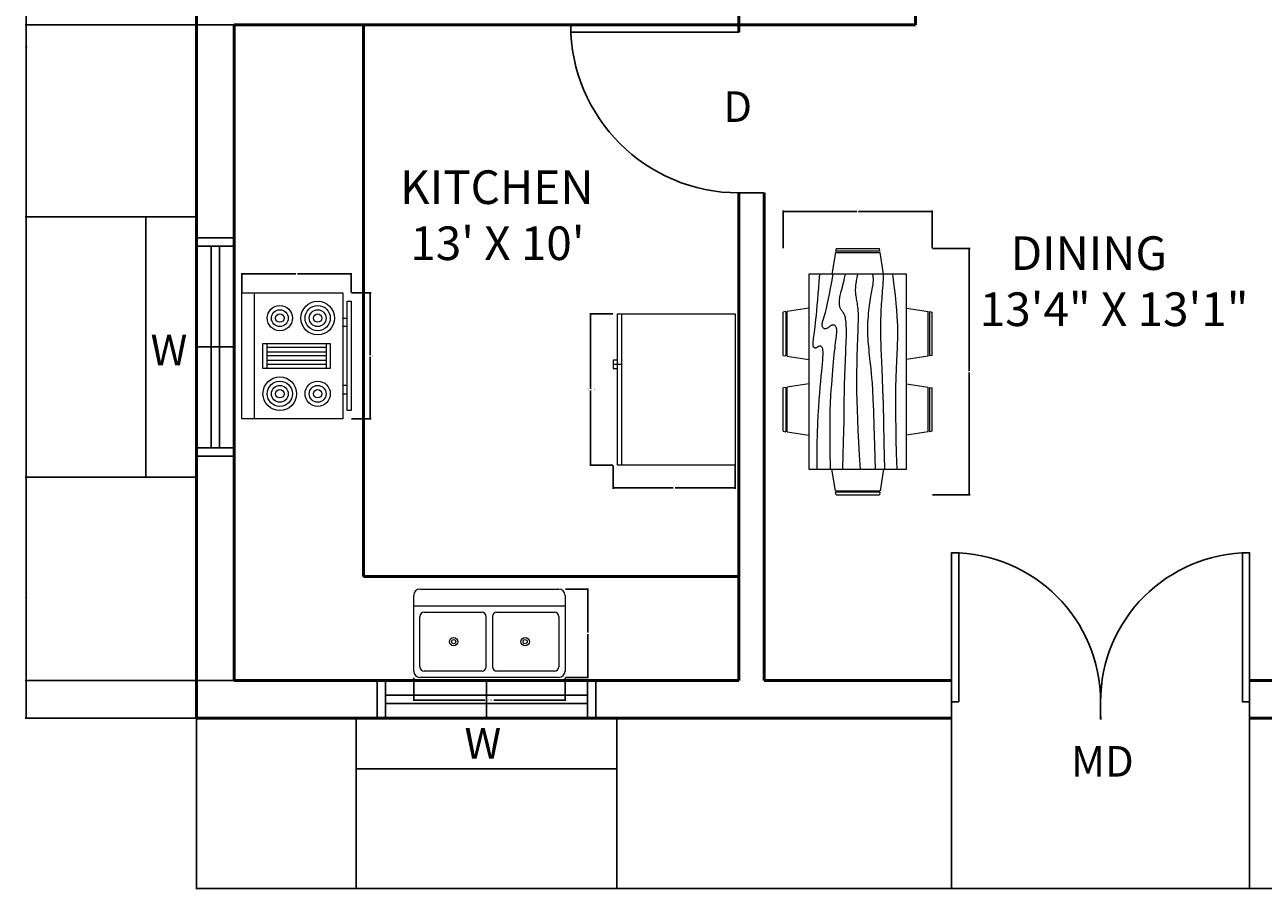
# Model space of a CAD drawing. Units: inches. Extents: x -73 to 1162, y -188 to 590.
# Tile 1 of 9: x -73 to 222, y -188 to 17. Entities that reach past the tile are written whole.
import ezdxf

# ---------------------------------------------------------------- set-up
doc = ezdxf.new("R2010")
doc.units = ezdxf.units.IN
doc.header["$MEASUREMENT"] = 0
for name, color, linetype, lineweight in [('A-ANNO-DIMS', 2, 'Continuous', 18), ('A-ANNO-TEXT', 7, 'Continuous', 25), ('A-AREA-IDEN', 2, 'Continuous', 25), ('A-DOOR', 3, 'Continuous', 25), ('A-FLOR-FIXT', 8, 'Continuous', 18), ('A-FURN', 8, 'Continuous', 18), ('A-GLAZ', 4, 'Continuous', 25), ('A-WALL', 7, 'Continuous', 50)]:
    doc.layers.add(name, color=color, linetype=linetype, lineweight=lineweight)
doc.styles.get("Standard").update_dxf_attribs({"font": 'arial.ttf'})
doc.dimstyles.get("Standard").update_dxf_attribs({"dimtxt": 0.18, "dimasz": 0.18, "dimexe": 0.18, "dimexo": 0.0625, "dimgap": 0.09, "dimtad": 0, "dimtih": 1, "dimtoh": 1, "dimdec": 1, "dimzin": 0, "dimdsep": 46, "dimlunit": 4, "dimtxsty": 'Standard', "dimcen": 0.09, "dimadec": 0, "dimazin": 0, "dimtfac": 1, "dimtdec": 1, "dimtofl": 0, "dimtmove": 0, "dimatfit": 3, "dimfxl": 1, "dimtolj": 1, "dimtzin": 0, "dimarcsym": 0})

# ---------------------------------------------------------------- blocks, each defined once
blk = doc.blocks.new('*U6')
for p, q in [((0, 0), (0, -6)), ((-40, 0), (-40, -6))]:
    blk.add_line(p, q)
blk.add_lwpolyline([(0, 0), (0, 40), (-1.75, 40), (-1.75, 0)], close=True)
blk.add_arc((0, 0), 40, 90, 180)
blk = doc.blocks.new('*U4')
for p, q in [((0, 0), (0, -100)), ((900, 0), (900, -100))]:
    blk.add_line(p, q)
blk.add_lwpolyline([(0, 0), (0, 900), (43.75, 900), (43.75, 0)], close=True)
blk.add_arc((0, 0), 900, 0, 90)
blk = doc.blocks.new('Dining Set - 36 x 72 in.')
for p, q in [((-22, 27.5), (-22.1562, 26.50042)), ((-22, 27.5), (-6, 27.5)), ((-5.8437, 26.49966), (-6, 27.5)), ((6, 27.5), (5.8438, 26.50042)), ((6, 27.5), (22, 27.5)), ((22.1563, 26.49966), (22, 27.5)), ((-22.2343, 26.00059), (-23.4847, 17.99762)), ((-22.2304, 26), (-5.7608, 26)), ((-5.8416, 26.5), (-22.1534, 26.5)), ((-4.5152, 17.99762), (-5.7655, 25.99926)), ((5.7657, 26.00059), (4.5153, 17.99762)), ((5.7696, 26), (22.2392, 26)), ((22.1584, 26.5), (5.8466, 26.5)), ((23.4848, 17.99762), (22.2345, 25.99926)), ((36, 18), (-36, 18)), ((-36, 18), (-36, -18)), ((36, -18), (36, 18)), ((-44.0006, 8.23428), (-35.9976, 9.48474)), ((44.0006, 8.23428), (35.9976, 9.48474)), ((-45.5, 8), (-44.5004, 8.15617)), ((-45.5, 8), (-45.5, -8)), ((-44.5, -8.15843), (-44.5, 8.15338)), ((-44, 8.23041), (-44, -8.23915)), ((44, 8.23041), (44, -8.23915)), ((44.5, -8.15843), (44.5, 8.15338)), ((45.5, 8), (44.5005, 8.15617)), ((45.5, 8), (45.5, -8)), ((-44.4997, -8.15631), (-45.5, -8)), ((-35.9976, -9.48476), (-43.9993, -8.2345)), ((35.9976, -9.48476), (43.9993, -8.2345)), ((44.4997, -8.15631), (45.5, -8)), ((-36, -18), (36, -18)), ((-22.2343, -26.0006), (-23.4847, -17.99762)), ((-4.5152, -17.99762), (-5.7655, -25.99928)), ((5.7657, -26.0006), (4.5153, -17.99762)), ((23.4848, -17.99762), (22.2345, -25.99928)), ((-22.2304, -26), (-5.7608, -26)), ((-22, -27.5), (-22.1562, -26.50044)), ((-5.8416, -26.5), (-22.1534, -26.5)), ((-5.8437, -26.49967), (-6, -27.5)), ((5.7696, -26), (22.2392, -26)), ((6, -27.5), (5.8438, -26.50044)), ((22.1584, -26.5), (5.8466, -26.5)), ((22.1563, -26.49967), (22, -27.5)), ((-22, -27.5), (-6, -27.5)), ((6, -27.5), (22, -27.5))]:
    blk.add_line(p, q)
for points in [[(-36, 15), (-31.1772, 14.97754), (-26.8079, 14.91406), (-22.8538, 14.81543), (-19.276, 14.6875), (-16.0362, 14.53613), (-13.0957, 14.36718), (-10.4159, 14.18652), (-7.9583, 14), (-5.6904, 13.81315), (-3.6035, 13.63021), (-1.6954, 13.45508), (0.0365, 13.29166), (1.5945, 13.14388), (2.9811, 13.01562), (4.1988, 12.9108), (5.25, 12.83333), (6.1393, 12.78613), (6.8802, 12.76823), (7.4883, 12.77767), (7.9792, 12.8125), (8.3685, 12.87077), (8.6719, 12.95052), (8.9049, 13.0498), (9.0833, 13.16666), (9.2205, 13.29899), (9.3216, 13.44401), (9.3895, 13.59879), (9.4271, 13.76041), (9.4373, 13.92594), (9.4232, 14.09245), (9.3875, 14.257), (9.3333, 14.41666), (9.2638, 14.56917), (9.1836, 14.71484), (9.0975, 14.85465), (9.0104, 14.98958), (8.9272, 15.1206), (8.8529, 15.2487), (8.7922, 15.37483), (8.75, 15.5), (8.7305, 15.62467), (8.7344, 15.74739), (8.7617, 15.86621), (8.8125, 15.97916), (8.8867, 16.08431), (8.9844, 16.17968), (9.1055, 16.26334), (9.25, 16.33333), (9.4189, 16.38802), (9.6172, 16.42708), (9.8506, 16.45052), (10.125, 16.45833), (10.4463, 16.45052), (10.8203, 16.42708), (11.2529, 16.38802), (11.75, 16.33333), (12.3184, 16.26318), (12.9694, 16.17838), (13.7151, 16.07991), (14.5677, 15.96875), (15.5395, 15.84586), (16.6426, 15.71224), (17.8893, 15.56884), (19.2917, 15.41666), (20.859, 15.25667), (22.5879, 15.08984), (24.4721, 14.91715), (26.5052, 14.73958), (28.6809, 14.5581), (30.9929, 14.3737), (33.4347, 14.18733), (36, 14)], [(-36, 10), (-28.9766, 10.14274), (-23.1725, 10.20442), (-18.4241, 10.19775), (-14.5677, 10.13541), (-11.4399, 10.03011), (-8.877, 9.89453), (-6.7154, 9.74137), (-4.7917, 9.58333), (-2.9698, 9.43082), (-1.2246, 9.28515), (0.4415, 9.14534), (2.026, 9.01041), (3.5266, 8.87939), (4.9408, 8.7513), (6.266, 8.62516), (7.5, 8.5), (8.6411, 8.37549), (9.6914, 8.2539), (10.6538, 8.13818), (11.5312, 8.03125), (12.3267, 7.93603), (13.043, 7.85547), (13.6831, 7.79248), (14.25, 7.75), (14.7471, 7.7303), (15.1797, 7.73307), (15.5537, 7.75732), (15.875, 7.80208), (16.1494, 7.86637), (16.3828, 7.94922), (16.5811, 8.04964), (16.75, 8.16666), (16.8944, 8.29915), (17.0143, 8.44531), (17.1089, 8.60319), (17.1771, 8.77083), (17.218, 8.94629), (17.2305, 9.1276), (17.2137, 9.31282), (17.1667, 9.5), (17.0895, 9.6875), (16.987, 9.875), (16.8649, 10.0625), (16.7292, 10.25), (16.5856, 10.4375), (16.4401, 10.625), (16.2985, 10.8125), (16.1667, 11), (16.05, 11.18733), (15.9518, 11.3737), (15.8752, 11.5581), (15.8229, 11.73958), (15.798, 11.91715), (15.8034, 12.08984), (15.842, 12.25667), (15.9167, 12.41666), (16.0295, 12.56836), (16.1784, 12.70833), (16.3605, 12.83268), (16.5729, 12.9375), (16.8127, 13.01888), (17.0768, 13.07291), (17.3625, 13.0957), (17.6667, 13.08333), (17.9894, 13.03312), (18.3418, 12.94726), (18.7382, 12.82918), (19.1927, 12.68229), (19.7195, 12.51001), (20.3327, 12.31575), (21.0465, 12.10294), (21.875, 11.875), (22.8357, 11.63354), (23.959, 11.37304), (25.2786, 11.08618), (26.8282, 10.76562), (28.6414, 10.40405), (30.752, 9.99414), (33.1936, 9.52856), (36, 9)], [(-36, 5.5), (-30.7157, 5.3348), (-26.069, 5.20963), (-21.9946, 5.11767), (-18.4271, 5.05208), (-15.3009, 5.00602), (-12.5508, 4.97265), (-10.1112, 4.94515), (-7.9167, 4.91666), (-5.909, 4.88167), (-4.0586, 4.83984), (-2.3429, 4.79215), (-0.7396, 4.73958), (0.7739, 4.6831), (2.22, 4.6237), (3.6213, 4.56233), (5, 4.5), (6.373, 4.43782), (7.7344, 4.3776), (9.0723, 4.32129), (10.375, 4.27083), (11.6309, 4.22819), (12.8281, 4.19531), (13.9551, 4.17415), (15, 4.16666), (15.954, 4.17448), (16.819, 4.19791), (17.6001, 4.23698), (18.3021, 4.29166), (18.9299, 4.36198), (19.4883, 4.44791), (19.9823, 4.54948), (20.4167, 4.66666), (20.7969, 4.79899), (21.1302, 4.94401), (21.4245, 5.09879), (21.6875, 5.26041), (21.9271, 5.42594), (22.1511, 5.59245), (22.3672, 5.757), (22.5834, 5.91666), (22.8065, 6.06868), (23.0404, 6.21093), (23.2879, 6.34147), (23.5521, 6.45833), (23.8358, 6.55957), (24.142, 6.64323), (24.4735, 6.70735), (24.8334, 6.75), (25.2235, 6.76969), (25.642, 6.76692), (26.0858, 6.74267), (26.5521, 6.69791), (27.0379, 6.63362), (27.5404, 6.55078), (28.0565, 6.45036), (28.5834, 6.33333), (29.1242, 6.19987), (29.7071, 6.04687), (30.3661, 5.87044), (31.1354, 5.66666), (32.0493, 5.43164), (33.142, 5.16146), (34.4475, 4.85221), (36, 4.5)], [(-36, -1), (-30.7915, -0.6591), (-26.0195, -0.38216), (-21.6519, -0.16284), (-17.6563, 0.00521), (-14.0005, 0.12833), (-10.6523, 0.21289), (-7.5796, 0.26522), (-4.75, 0.29166), (-2.134, 0.29793), (0.2878, 0.28711), (2.5317, 0.26163), (4.6146, 0.22396), (6.5529, 0.17651), (8.3633, 0.12174), (10.0623, 0.06209), (11.6667, 0), (13.1899, -0.06201), (14.6341, -0.1211), (15.9982, -0.17432), (17.2813, -0.21875), (18.4823, -0.25147), (19.6003, -0.26953), (20.6343, -0.27002), (21.5834, -0.25), (22.4481, -0.20768), (23.2357, -0.14584), (23.9549, -0.06836), (24.6146, 0.02083), (25.2235, 0.11784), (25.7904, 0.21875), (26.3241, 0.31966), (26.8334, 0.41666), (27.3265, 0.50618), (27.8099, 0.58593), (28.2894, 0.65397), (28.7709, 0.70833), (29.2601, 0.74707), (29.763, 0.76823), (30.2855, 0.76985), (30.8334, 0.75), (31.4088, 0.70784), (31.9994, 0.64713), (32.589, 0.57275), (33.1615, 0.48958), (33.7008, 0.4025), (34.1908, 0.3164), (34.6153, 0.23616), (34.9584, 0.16666), (35.2099, 0.11165), (35.3848, 0.07031), (35.504, 0.04069), (35.5886, 0.02083), (35.6594, 0.00879), (35.7377, 0.0026), (35.8442, 0.00032), (36, 0)], [(-36, -6.5), (-27.1843, -6.31267), (-20.084, -6.1263), (-14.469, -5.9419), (-10.1094, -5.76042), (-6.7752, -5.58285), (-4.2363, -5.41016), (-2.2629, -5.24333), (-0.625, -5.08334), (0.8708, -4.93099), (2.2715, -4.78646), (3.5872, -4.64974), (4.8281, -4.52084), (6.0046, -4.39974), (7.127, -4.28646), (8.2053, -4.18099), (9.25, -4.08334), (10.2705, -3.99382), (11.2734, -3.91407), (12.2647, -3.84603), (13.25, -3.79167), (14.2354, -3.75293), (15.2266, -3.73177), (16.2295, -3.73015), (17.25, -3.75), (18.2912, -3.79248), (19.3451, -3.85547), (20.4009, -3.93604), (21.4479, -4.03125), (22.4754, -4.13819), (23.4727, -4.25391), (24.4289, -4.37549), (25.3334, -4.5), (26.1785, -4.62492), (26.9694, -4.74935), (27.7145, -4.87281), (28.4219, -4.99479), (29.1, -5.11483), (29.7572, -5.23242), (30.4016, -5.34709), (31.0417, -5.45834), (31.6837, -5.56437), (32.3262, -5.65821), (32.9658, -5.73153), (33.599, -5.77604), (34.2224, -5.78345), (34.8327, -5.74545), (35.4264, -5.65373), (36, -5.5)], [(-36, -10), (-26.4022, -9.81299), (-18.4675, -9.62891), (-11.9839, -9.45069), (-6.7396, -9.28125), (-2.5226, -9.12354), (0.8789, -8.98047), (3.6769, -8.85498), (6.0833, -8.75), (8.2767, -8.66765), (10.3021, -8.60677), (12.1712, -8.56543), (13.8958, -8.54167), (15.4876, -8.53353), (16.9583, -8.53907), (18.3197, -8.55632), (19.5834, -8.58334), (20.7616, -8.61841), (21.8685, -8.66081), (22.9188, -8.71004), (23.9271, -8.76563), (24.9081, -8.82707), (25.8763, -8.89388), (26.8465, -8.96558), (27.8334, -9.04167), (28.8474, -9.12118), (29.8828, -9.20117), (30.93, -9.27824), (31.9792, -9.34896), (33.0205, -9.40991), (34.0443, -9.45768), (35.0407, -9.48885), (36, -9.5)], [(-36, -14.5), (-30.0881, -14.33513), (-25.0332, -14.21224), (-20.7312, -14.12647), (-17.0781, -14.07292), (-13.97, -14.04671), (-11.3027, -14.04297), (-8.9724, -14.05681), (-6.875, -14.08334), (-4.9224, -14.11833), (-3.0905, -14.16016), (-1.3709, -14.20785), (0.2448, -14.26042), (1.7647, -14.3169), (3.1973, -14.3763), (4.5507, -14.43767), (5.8333, -14.5), (7.0554, -14.5621), (8.235, -14.62175), (9.3922, -14.67652), (10.5469, -14.72396), (11.7192, -14.76164), (12.929, -14.78711), (14.1965, -14.79794), (15.5417, -14.79167), (16.9933, -14.76424), (18.6152, -14.70508), (20.4804, -14.60197), (22.6615, -14.44271), (25.2312, -14.21509), (28.2624, -13.9069), (31.8277, -13.50594), (36, -13)]]:
    blk.add_lwpolyline(points)
blk = doc.blocks.new('Range-Oven - 30 in top')
for p, q in [((0, -3), (30, -3)), ((12, -6), (18, -6)), ((13, -20), (13, -6)), ((14, -6), (14, -20)), ((15, -20), (15, -6)), ((16, -6), (16, -20)), ((17, -20), (17, -6)), ((18, -20), (12, -20)), ((6, -24), (6, -25)), ((8, -25), (8, -24)), ((22, -25), (22, -24)), ((24, -24), (24, -25))]:
    blk.add_line(p, q)
for points in [[(0, -24), (0, 0), (30, 0), (30, -24)], [(12, -21), (12, -5), (18, -5), (18, -21)], [(2, -26), (2, -25), (28, -25), (28, -26)]]:
    blk.add_lwpolyline(points, close=True)
for centre, radius in [((6, -9), 4), ((6, -9), 3), ((6, -9), 2), ((6, -9), 1), ((24, -9), 3), ((24, -9), 2), ((24, -9), 1), ((24, -18), 4), ((6, -18), 3), ((6, -18), 2), ((6, -18), 1), ((24, -18), 3), ((24, -18), 2), ((24, -18), 1)]:
    blk.add_circle(centre, radius)
blk = doc.blocks.new('Sink-double - 36 in top')
for p, q in [((-18, -4), (18, -4)), ((-0.75, -18.5), (-0.75, -6.5)), ((0.75, -6.5), (0.75, -18.5))]:
    blk.add_line(p, q)
for points in [[(-16.5, 0), (16.5, 0)], [(-18, -19.5), (-18, -1.5)], [(18, -1.5), (18, -19.5)], [(-15.5, -5.5), (-1.75, -5.5)], [(1.75, -5.5), (15.5, -5.5)], [(-16.5, -18.5), (-16.5, -6.5)], [(16.5, -6.5), (16.5, -18.5)], [(-1.75, -19.5), (-15.5, -19.5)], [(15.5, -19.5), (1.75, -19.5)], [(16.5, -21), (-16.5, -21)]]:
    blk.add_lwpolyline(points)
for centre, radius in [((-8.5, -12.5), 1), ((8.5, -12.5), 1), ((-8.5, -12.5), 0.5), ((8.5, -12.5), 0.5)]:
    blk.add_circle(centre, radius)
for centre, radius, start, end in [((-16.5, -1.5), 1.5, 90, 180), ((16.5, -1.5), 1.5, 0, 90), ((-15.5, -6.5), 1, 90, 180), ((-1.75, -6.5), 1, 0, 90), ((1.75, -6.5), 1, 90, 180), ((15.5, -6.5), 1, 0, 90), ((-16.5, -19.5), 1.5, 180, 270), ((-15.5, -18.5), 1, 180, 270), ((-1.75, -18.5), 1, 270, 0), ((1.75, -18.5), 1, 180, 270), ((15.5, -18.5), 1, 270, 0), ((16.5, -19.5), 1.5, 270, 0)]:
    blk.add_arc(centre, radius, start, end)
blk = doc.blocks.new('Refrigerator-2 door - 36 in top')
for p, q in [((0, -26.999999), (36, -26.999999)), ((11, -27.999999), (11, -28.999999)), ((11, -28.999999), (13, -28.999999)), ((12, -26.999999), (12, -28.999999)), ((13, -28.999999), (13, -27.999999))]:
    blk.add_line(p, q)
blk.add_lwpolyline([(0, -27.999999), (0, 0), (36, 0), (36, -27.999999)], close=True)
blk = doc.blocks.new('WIN-W')
for p, q in [((9, 57), (9, 62)), ((9, 62), (21, 62)), ((21, 62), (21, 0)), ((0, 57), (9, 57)), ((0, 5), (9, 5)), ((9, 5), (9, 0)), ((9, 0), (21, 0))]:
    blk.add_line(p, q)
blk = doc.blocks.new('*D40')
at = {"layer": 'A-ANNO-DIMS', "color": 0, "lineweight": -2, "transparency": 16777216}
for p, q in [((143.21, -36.02), (152.13, -36.02)), ((151.95, -36.2), (151.95, -65.17)), ((151.95, -94.51), (151.95, -65.54)), ((143.21, -94.69), (152.13, -94.69))]:
    blk.add_line(p, q, dxfattribs=at)
at = {"layer": 'A-ANNO-DIMS', "color": 0, "transparency": 16777216}
for points in [[(151.92, -36.2), (151.98, -36.2), (151.95, -36.02)], [(151.92, -94.51), (151.98, -94.51), (151.95, -94.69)]]:
    blk.add_solid(points, dxfattribs=at)
at = {"layer": 'Defpoints', "color": 0, "transparency": 16777216}
for p in [(143.15, -36.02), (151.95, -36.02), (143.15, -94.69)]:
    blk.add_point(p, dxfattribs=at)
at = {"layer": 'A-ANNO-DIMS', "color": 0, "transparency": 16777216, "insert": (151.95, -65.35), "char_height": 0.18, "attachment_point": 5}
blk.add_mtext('\\A1;DINING SET 59', dxfattribs=at)
blk = doc.blocks.new('*D41')
at = {"layer": 'A-ANNO-DIMS', "color": 0, "lineweight": -2, "transparency": 16777216}
for p, q in [((107.69, -35.96), (107.69, -27.04)), ((107.87, -27.22), (125.2, -27.22)), ((142.97, -27.22), (125.64, -27.22)), ((143.15, -35.96), (143.15, -27.04))]:
    blk.add_line(p, q, dxfattribs=at)
at = {"layer": 'A-ANNO-DIMS', "color": 0, "transparency": 16777216}
for points in [[(107.87, -27.19), (107.87, -27.25), (107.69, -27.22)], [(142.97, -27.19), (142.97, -27.25), (143.15, -27.22)]]:
    blk.add_solid(points, dxfattribs=at)
at = {"layer": 'Defpoints', "color": 0, "transparency": 16777216}
for p in [(107.69, -27.22), (107.69, -36.02), (143.15, -36.02)]:
    blk.add_point(p, dxfattribs=at)
at = {"layer": 'A-ANNO-DIMS', "color": 0, "transparency": 16777216, "insert": (125.42, -27.22), "char_height": 0.18, "attachment_point": 5}
blk.add_mtext('\\A1;35', dxfattribs=at)
blk = doc.blocks.new('*D46')
at = {"layer": 'A-ANNO-DIMS', "color": 0, "lineweight": -2, "transparency": 16777216}
for p, q in [((5.07, -46.61), (9.69, -46.61)), ((9.51, -46.79), (9.51, -61.43)), ((9.51, -76.43), (9.51, -61.8)), ((5.07, -76.61), (9.69, -76.61))]:
    blk.add_line(p, q, dxfattribs=at)
at = {"layer": 'A-ANNO-DIMS', "color": 0, "transparency": 16777216}
for points in [[(9.48, -46.79), (9.54, -46.79), (9.51, -46.61)], [(9.48, -76.43), (9.54, -76.43), (9.51, -76.61)]]:
    blk.add_solid(points, dxfattribs=at)
at = {"layer": 'Defpoints', "color": 0, "transparency": 16777216}
for p in [(5.01, -46.61), (9.51, -46.61), (5.01, -76.61)]:
    blk.add_point(p, dxfattribs=at)
at = {"layer": 'A-ANNO-DIMS', "color": 0, "transparency": 16777216, "insert": (9.51, -61.61), "char_height": 0.18, "attachment_point": 5}
blk.add_mtext('\\A1;RANGE 30', dxfattribs=at)
blk = doc.blocks.new('*D47')
at = {"layer": 'A-ANNO-DIMS', "color": 0, "lineweight": -2, "transparency": 16777216}
for p, q in [((-20.99, -46.55), (-20.99, -41.93)), ((-20.81, -42.11), (-8.21, -42.11)), ((4.83, -42.11), (-7.77, -42.11)), ((5.01, -46.55), (5.01, -41.93))]:
    blk.add_line(p, q, dxfattribs=at)
at = {"layer": 'A-ANNO-DIMS', "color": 0, "transparency": 16777216}
for points in [[(-20.81, -42.08), (-20.81, -42.14), (-20.99, -42.11)], [(4.83, -42.08), (4.83, -42.14), (5.01, -42.11)]]:
    blk.add_solid(points, dxfattribs=at)
at = {"layer": 'Defpoints', "color": 0, "transparency": 16777216}
for p in [(-20.99, -42.11), (-20.99, -46.61), (5.01, -46.61)]:
    blk.add_point(p, dxfattribs=at)
at = {"layer": 'A-ANNO-DIMS', "color": 0, "transparency": 16777216, "insert": (-7.99, -42.11), "char_height": 0.18, "attachment_point": 5}
blk.add_mtext('\\A1;26', dxfattribs=at)
blk = doc.blocks.new('*D48')
at = {"layer": 'A-ANNO-DIMS', "color": 0, "lineweight": -2, "transparency": 16777216}
for p, q in [((19.84, -138.16), (19.84, -143.67)), ((55.84, -138.16), (55.84, -143.67)), ((20.02, -143.49), (36.74, -143.49)), ((55.66, -143.49), (38.93, -143.49))]:
    blk.add_line(p, q, dxfattribs=at)
at = {"layer": 'A-ANNO-DIMS', "color": 0, "transparency": 16777216}
for points in [[(20.02, -143.46), (20.02, -143.52), (19.84, -143.49)], [(55.66, -143.46), (55.66, -143.52), (55.84, -143.49)]]:
    blk.add_solid(points, dxfattribs=at)
at = {"layer": 'Defpoints', "color": 0, "transparency": 16777216}
for p in [(19.84, -138.09), (55.84, -138.09), (55.84, -143.49)]:
    blk.add_point(p, dxfattribs=at)
at = {"layer": 'A-ANNO-DIMS', "color": 0, "transparency": 16777216, "insert": (37.84, -143.49), "char_height": 0.18, "attachment_point": 5}
blk.add_mtext('\\A1;DOUBLE SINK 36', dxfattribs=at)
blk = doc.blocks.new('*D49')
at = {"layer": 'A-ANNO-DIMS', "color": 0, "lineweight": -2, "transparency": 16777216}
for p, q in [((55.9, -117.09), (61.42, -117.09)), ((61.24, -117.27), (61.24, -127.41)), ((61.24, -137.91), (61.24, -127.77)), ((55.9, -138.09), (61.42, -138.09))]:
    blk.add_line(p, q, dxfattribs=at)
at = {"layer": 'A-ANNO-DIMS', "color": 0, "transparency": 16777216}
for points in [[(61.21, -117.27), (61.27, -117.27), (61.24, -117.09)], [(61.21, -137.91), (61.27, -137.91), (61.24, -138.09)]]:
    blk.add_solid(points, dxfattribs=at)
at = {"layer": 'Defpoints', "color": 0, "transparency": 16777216}
for p in [(55.84, -117.09), (61.24, -117.09), (55.84, -138.09)]:
    blk.add_point(p, dxfattribs=at)
at = {"layer": 'A-ANNO-DIMS', "color": 0, "transparency": 16777216, "insert": (61.24, -127.59), "char_height": 0.18, "attachment_point": 5}
blk.add_mtext('\\A1;21', dxfattribs=at)
blk = doc.blocks.new('*D50')
at = {"layer": 'A-ANNO-DIMS', "color": 0, "lineweight": -2, "transparency": 16777216}
for p, q in [((67.21, -51.63), (61.7, -51.63)), ((61.88, -51.81), (61.88, -69.45)), ((61.88, -87.45), (61.88, -69.82)), ((67.21, -87.63), (61.7, -87.63))]:
    blk.add_line(p, q, dxfattribs=at)
at = {"layer": 'A-ANNO-DIMS', "color": 0, "transparency": 16777216}
for points in [[(61.85, -51.81), (61.91, -51.81), (61.88, -51.63)], [(61.85, -87.45), (61.91, -87.45), (61.88, -87.63)]]:
    blk.add_solid(points, dxfattribs=at)
at = {"layer": 'Defpoints', "color": 0, "transparency": 16777216}
for p in [(67.28, -51.63), (61.88, -87.63), (67.28, -87.63)]:
    blk.add_point(p, dxfattribs=at)
at = {"layer": 'A-ANNO-DIMS', "color": 0, "transparency": 16777216, "insert": (61.88, -69.63), "char_height": 0.18, "attachment_point": 5}
blk.add_mtext('\\A1;REFRIGERATOR 36', dxfattribs=at)
blk = doc.blocks.new('*D51')
at = {"layer": 'A-ANNO-DIMS', "color": 0, "lineweight": -2, "transparency": 16777216}
for p, q in [((67.28, -87.69), (67.28, -93.21)), ((96.28, -87.69), (96.28, -93.21)), ((67.46, -93.03), (81.55, -93.03)), ((96.1, -93.03), (82, -93.03))]:
    blk.add_line(p, q, dxfattribs=at)
at = {"layer": 'A-ANNO-DIMS', "color": 0, "transparency": 16777216}
for points in [[(67.46, -93), (67.46, -93.06), (67.28, -93.03)], [(96.1, -93), (96.1, -93.06), (96.28, -93.03)]]:
    blk.add_solid(points, dxfattribs=at)
at = {"layer": 'Defpoints', "color": 0, "transparency": 16777216}
for p in [(67.28, -87.63), (96.28, -87.63), (96.28, -93.03)]:
    blk.add_point(p, dxfattribs=at)
at = {"layer": 'A-ANNO-DIMS', "color": 0, "transparency": 16777216, "insert": (81.78, -93.03), "char_height": 0.18, "attachment_point": 5}
blk.add_mtext('\\A1;29', dxfattribs=at)
blk = doc.blocks.new('*D58')
at = {"layer": 'A-ANNO-DIMS', "color": 0, "lineweight": -2, "transparency": 16777216}
for p, q in [((-31.83, -147.88), (-31.83, -188.5)), ((501.17, -147.88), (501.17, -188.5)), ((-31.65, -188.32), (234.38, -188.32)), ((500.99, -188.32), (234.96, -188.32))]:
    blk.add_line(p, q, dxfattribs=at)
at = {"layer": 'A-ANNO-DIMS', "color": 0, "transparency": 16777216}
for points in [[(-31.65, -188.29), (-31.65, -188.35), (-31.83, -188.32)], [(500.99, -188.29), (500.99, -188.35), (501.17, -188.32)]]:
    blk.add_solid(points, dxfattribs=at)
at = {"layer": 'Defpoints', "color": 0, "transparency": 16777216}
for p in [(-31.83, -147.82), (501.17, -147.82), (501.17, -188.32)]:
    blk.add_point(p, dxfattribs=at)
at = {"layer": 'A-ANNO-DIMS', "color": 0, "transparency": 16777216, "insert": (234.67, -188.32), "char_height": 0.18, "attachment_point": 5}
blk.add_mtext('\\A1;533', dxfattribs=at)
blk = doc.blocks.new('*D65')
at = {"layer": 'A-ANNO-DIMS', "color": 0, "lineweight": -2, "transparency": 16777216}
for p, q in [((-31.89, 152.18), (-72.51, 152.18)), ((-72.33, 152), (-72.33, 2.37)), ((-72.33, -147.64), (-72.33, 2)), ((-31.89, -147.82), (-72.51, -147.82))]:
    blk.add_line(p, q, dxfattribs=at)
at = {"layer": 'A-ANNO-DIMS', "color": 0, "transparency": 16777216}
for points in [[(-72.36, 152), (-72.3, 152), (-72.33, 152.18)], [(-72.36, -147.64), (-72.3, -147.64), (-72.33, -147.82)]]:
    blk.add_solid(points, dxfattribs=at)
at = {"layer": 'Defpoints', "color": 0, "transparency": 16777216}
for p in [(-31.83, 152.18), (-72.33, -147.82), (-31.83, -147.82)]:
    blk.add_point(p, dxfattribs=at)
at = {"layer": 'A-ANNO-DIMS', "color": 0, "transparency": 16777216, "insert": (-72.33, 2.18), "char_height": 0.18, "attachment_point": 5}
blk.add_mtext('\\A1;300', dxfattribs=at)
blk = doc.blocks.new('*D67')
at = {"layer": 'A-ANNO-DIMS', "color": 0, "lineweight": -2, "transparency": 16777216}
for p, q in [((-43.89, 52.18), (-72.51, 52.18)), ((-72.33, 52), (-72.33, 12.04)), ((-72.33, -28.3), (-72.33, 11.67)), ((-43.89, -28.48), (-72.51, -28.48))]:
    blk.add_line(p, q, dxfattribs=at)
at = {"layer": 'A-ANNO-DIMS', "color": 0, "transparency": 16777216}
for points in [[(-72.36, 52), (-72.3, 52), (-72.33, 52.18)], [(-72.36, -28.3), (-72.3, -28.3), (-72.33, -28.48)]]:
    blk.add_solid(points, dxfattribs=at)
at = {"layer": 'Defpoints', "color": 0, "transparency": 16777216}
for p in [(-43.83, 52.18), (-72.33, -28.48), (-43.83, -28.48)]:
    blk.add_point(p, dxfattribs=at)
at = {"layer": 'A-ANNO-DIMS', "color": 0, "transparency": 16777216, "insert": (-72.33, 11.85), "char_height": 0.18, "attachment_point": 5}
blk.add_mtext('\\A1;80.66', dxfattribs=at)
blk = doc.blocks.new('*D68')
at = {"layer": 'A-ANNO-DIMS', "color": 0, "lineweight": -2, "transparency": 16777216}
for p, q in [((-43.89, -90.48), (-72.51, -90.48)), ((-72.33, -90.66), (-72.33, -118.96)), ((-72.33, -147.64), (-72.33, -119.33)), ((-31.89, -147.82), (-72.51, -147.82))]:
    blk.add_line(p, q, dxfattribs=at)
at = {"layer": 'A-ANNO-DIMS', "color": 0, "transparency": 16777216}
for points in [[(-72.36, -90.66), (-72.3, -90.66), (-72.33, -90.48)], [(-72.36, -147.64), (-72.3, -147.64), (-72.33, -147.82)]]:
    blk.add_solid(points, dxfattribs=at)
at = {"layer": 'Defpoints', "color": 0, "transparency": 16777216}
for p in [(-43.83, -90.48), (-72.33, -147.82), (-31.83, -147.82)]:
    blk.add_point(p, dxfattribs=at)
at = {"layer": 'A-ANNO-DIMS', "color": 0, "transparency": 16777216, "insert": (-72.33, -119.15), "char_height": 0.18, "attachment_point": 5}
blk.add_mtext('\\A1;57.34', dxfattribs=at)
blk = doc.blocks.new('*D69')
at = {"layer": 'A-ANNO-DIMS', "color": 0, "lineweight": -2, "transparency": 16777216}
for p, q in [((-31.83, -147.88), (-31.83, -188.5)), ((6.17, -159.88), (6.17, -188.5)), ((-31.65, -188.32), (-13.05, -188.32)), ((5.99, -188.32), (-12.61, -188.32))]:
    blk.add_line(p, q, dxfattribs=at)
at = {"layer": 'A-ANNO-DIMS', "color": 0, "transparency": 16777216}
for points in [[(-31.65, -188.29), (-31.65, -188.35), (-31.83, -188.32)], [(5.99, -188.29), (5.99, -188.35), (6.17, -188.32)]]:
    blk.add_solid(points, dxfattribs=at)
at = {"layer": 'Defpoints', "color": 0, "transparency": 16777216}
for p in [(-31.83, -147.82), (6.17, -159.82), (6.17, -188.32)]:
    blk.add_point(p, dxfattribs=at)
at = {"layer": 'A-ANNO-DIMS', "color": 0, "transparency": 16777216, "insert": (-12.83, -188.32), "char_height": 0.18, "attachment_point": 5}
blk.add_mtext('\\A1;38', dxfattribs=at)
blk = doc.blocks.new('*D70')
at = {"layer": 'A-ANNO-DIMS', "color": 0, "lineweight": -2, "transparency": 16777216}
for p, q in [((147.74, -147.88), (147.74, -188.5)), ((68.17, -159.88), (68.17, -188.5)), ((68.35, -188.32), (107.56, -188.32)), ((147.56, -188.32), (108.35, -188.32))]:
    blk.add_line(p, q, dxfattribs=at)
at = {"layer": 'A-ANNO-DIMS', "color": 0, "transparency": 16777216}
for points in [[(68.35, -188.29), (68.35, -188.35), (68.17, -188.32)], [(147.56, -188.29), (147.56, -188.35), (147.74, -188.32)]]:
    blk.add_solid(points, dxfattribs=at)
at = {"layer": 'Defpoints', "color": 0, "transparency": 16777216}
for p in [(147.74, -147.82), (68.17, -159.82), (147.74, -188.32)]:
    blk.add_point(p, dxfattribs=at)
at = {"layer": 'A-ANNO-DIMS', "color": 0, "transparency": 16777216, "insert": (107.95, -188.32), "char_height": 0.18, "attachment_point": 5}
blk.add_mtext('\\A1;79.57', dxfattribs=at)
blk = doc.blocks.new('*D71')
at = {"layer": 'A-ANNO-DIMS', "color": 0, "lineweight": -2, "transparency": 16777216}
for p, q in [((147.74, -147.88), (147.74, -188.5)), ((218.6, -147.88), (218.6, -188.5)), ((147.92, -188.32), (182.78, -188.32)), ((218.42, -188.32), (183.56, -188.32))]:
    blk.add_line(p, q, dxfattribs=at)
at = {"layer": 'A-ANNO-DIMS', "color": 0, "transparency": 16777216}
for points in [[(147.92, -188.29), (147.92, -188.35), (147.74, -188.32)], [(218.42, -188.29), (218.42, -188.35), (218.6, -188.32)]]:
    blk.add_solid(points, dxfattribs=at)
at = {"layer": 'Defpoints', "color": 0, "transparency": 16777216}
for p in [(147.74, -147.82), (218.6, -147.82), (218.6, -188.32)]:
    blk.add_point(p, dxfattribs=at)
at = {"layer": 'A-ANNO-DIMS', "color": 0, "transparency": 16777216, "insert": (183.17, -188.32), "char_height": 0.18, "attachment_point": 5}
blk.add_mtext('\\A1;70.87', dxfattribs=at)
blk = doc.blocks.new('*D98')
at = {"layer": 'A-ANNO-DIMS', "color": 0, "lineweight": -2, "transparency": 16777216}
for p, q in [((-22.89, 17.18), (-72.51, 17.18)), ((-72.33, 17), (-72.33, -60.63)), ((-72.33, -138.64), (-72.33, -61)), ((-22.89, -138.82), (-72.51, -138.82))]:
    blk.add_line(p, q, dxfattribs=at)
at = {"layer": 'A-ANNO-DIMS', "color": 0, "transparency": 16777216}
for points in [[(-72.36, 17), (-72.3, 17), (-72.33, 17.18)], [(-72.36, -138.64), (-72.3, -138.64), (-72.33, -138.82)]]:
    blk.add_solid(points, dxfattribs=at)
at = {"layer": 'Defpoints', "color": 0, "transparency": 16777216}
for p in [(-72.33, 17.18), (-22.83, 17.18), (-22.83, -138.82)]:
    blk.add_point(p, dxfattribs=at)
at = {"layer": 'A-ANNO-DIMS', "color": 0, "transparency": 16777216, "insert": (-72.33, -60.82), "char_height": 0.18, "attachment_point": 5}
blk.add_mtext('\\A1;156', dxfattribs=at)

msp = doc.modelspace()

# ---------------------------------------------------------------- linework, layer by layer
at = {"layer": 'A-GLAZ'}
for p, q in [((-22.83, -35.4767), (-31.83, -35.4767)), ((-28.33, -83.4767), (-28.33, -35.4767)), ((-26.33, -83.4767), (-26.33, -35.4767)), ((-22.83, -59.4767), (-31.83, -59.4767)), ((-22.83, -83.4767), (-31.83, -83.4767)), ((13.17, -138.8156), (13.17, -147.8156)), ((37.17, -138.8156), (37.1411, -147.8155)), ((37.17, -138.8156), (37.17, -147.8156)), ((61.17, -138.8156), (61.17, -147.8156)), ((61.17, -142.3156), (13.17, -142.3156)), ((61.17, -144.3156), (13.17, -144.3156))]:
    msp.add_line(p, q, dxfattribs=at)
at = {"layer": 'A-WALL'}
for p, q in [((-31.83, 23.1844), (-31.83, -147.8156)), ((97.17, 15.4344), (97.17, 23.1844)), ((139.17, 23.1844), (139.17, 17.1844)), ((-22.83, 17.1844), (97.17, 17.1844)), ((-22.83, 17.1844), (-22.83, -138.8156)), ((7.9207, 17.1844), (7.9207, -114.0828)), ((97.17, 17.1844), (139.17, 17.1844)), ((97.17, -138.8156), (97.17, -22.8156)), ((103.17, -138.8156), (103.17, -22.8156)), ((7.9207, -114.0828), (97.17, -114.0828)), ((-22.83, -138.8156), (97.17, -138.8156)), ((103.17, -138.8156), (147.7369, -138.8156)), ((218.6031, -138.8156), (316.17, -138.8156)), ((-31.83, -147.8156), (103.17, -147.8156)), ((103.17, -147.8156), (147.7369, -147.8156)), ((182.9506, -147.8156), (183.3894, -147.8156)), ((218.6031, -147.8156), (501.17, -147.8156))]:
    msp.add_line(p, q, dxfattribs=at)

# ---------------------------------------------------------------- block references
at = {"layer": 'A-DOOR', "rotation": 90}
msp.add_blockref('*U6', (97.17, 17.1844), dxfattribs=at)
at = {"layer": 'A-DOOR', "yscale": 0.0393700787401575, "zscale": 0.0393700787401575}
for p, xscale in [((147.7369, -143.8785), 0.0393700787401575), ((218.6031, -143.8785), -0.0393700787401575)]:
    msp.add_blockref('*U4', p, dxfattribs=dict(at, xscale=xscale))
at = {"layer": 'A-FLOR-FIXT'}
for name, p, rotation in [('Range-Oven - 30 in top', (-20.9925, -76.6123), 90), ('Refrigerator-2 door - 36 in top', (96.2753, -51.6321), 270)]:
    msp.add_blockref(name, p, dxfattribs=dict(at, rotation=rotation))
msp.add_blockref('Sink-double - 36 in top', (37.8375, -117.0932), dxfattribs=at)
at = {"layer": 'A-FURN', "xscale": 0.6446915722569316, "yscale": 0.6446915722569316, "zscale": 0.6446915722569316, "rotation": 90}
msp.add_blockref('Dining Set - 36 x 72 in.', (125.4168, -65.3549), dxfattribs=at)
at = {"layer": 'A-GLAZ'}
for p, rotation in [((-22.83, -28.4763), 180), ((6.1696, -138.8156), 269.9999999999999)]:
    msp.add_blockref('WIN-W', p, dxfattribs=dict(at, rotation=rotation))

# ---------------------------------------------------------------- texts
at = {"layer": 'A-ANNO-TEXT'}
for s, height, p in [('D', 7.2829, (93.4554, -5.94)), ('W', 7.2829, (-42.7108, -63.8715)), ('W', 7.2829, (31.9183, -157.4009)), ('MD', 7.28289, (176.1454, -161.7))]:
    msp.add_text(s, height=height, dxfattribs=at).set_placement(p)
at = {"layer": 'A-AREA-IDEN', "char_height": 8, "attachment_point": 1}
for s, insert in [("KITCHEN\\P 13' X 10'", (16.5855, -17.461)), ('   DINING\\P13\'4" X 13\'1"', (154.4347, -33.1586))]:
    msp.add_mtext_dynamic_manual_height_columns(s, width=71.534965, gutter_width=1, heights=[0], dxfattribs=dict(at, insert=insert))

# ---------------------------------------------------------------- dimensions: what is measured, and where the dimension line sits
at = {"layer": 'A-ANNO-DIMS'}
for base, p1, p2, angle, override, picture, middle in [((-72.33, -147.8156), (-31.83, 152.1844), (-31.83, -147.8156), 90, {"dimdec": 0, "dimlfac": 1, "dimrnd": 0, "dimzin": 0, "dimdsep": 46, "dimlunit": 2}, '*D65', (-72.33, 2.1844)), ((-72.33, -28.4767), (-43.83, 52.1844), (-43.83, -28.4767), 90, {"dimdec": 2, "dimlfac": 1, "dimrnd": 0, "dimzin": 0, "dimdsep": 46, "dimlunit": 2}, '*D67', (-72.33, 11.8538)), ((-72.33, 17.1844), (-22.83, -138.8156), (-22.83, 17.1844), 90, {"dimdec": 0, "dimlfac": 1, "dimrnd": 0, "dimzin": 0, "dimdsep": 46, "dimlunit": 2}, '*D98', (-72.33, -60.8156)), ((107.6878, -27.2214), (143.1458, -36.0215), (107.6878, -36.0215), 180, {"dimdec": 0, "dimrnd": 0, "dimzin": 0, "dimlunit": 2}, '*D41', (125.4168, -27.2214)), ((-20.9925, -42.1123), (5.0075, -46.6123), (-20.9925, -46.6123), 180, {"dimdec": 0, "dimrnd": 0, "dimzin": 0, "dimlunit": 2}, '*D47', (-7.9925, -42.1123)), ((-72.33, -147.8156), (-43.83, -90.4767), (-31.83, -147.8156), 90, {"dimdec": 2, "dimlfac": 1, "dimrnd": 0, "dimzin": 0, "dimdsep": 46, "dimlunit": 2}, '*D68', (-72.33, -119.1462)), ((61.2375, -117.0932), (55.8375, -138.0932), (55.8375, -117.0932), 90, {"dimdec": 0, "dimrnd": 0, "dimzin": 0, "dimlunit": 2}, '*D49', (61.2375, -127.5932))]:
    dim = msp.add_linear_dim(base=base, p1=p1, p2=p2, angle=angle, dimstyle='Standard', override=override, dxfattribs=at)
    dim.commit()
    dim.dimension.update_dxf_attribs({"geometry": picture, "text_midpoint": middle})
for base, p1, p2, angle, text, picture, middle in [((151.9459, -36.0215), (143.1458, -94.6884), (143.1458, -36.0215), 90, 'DINING SET <>', '*D40', (151.9459, -65.3549)), ((9.5075, -46.6123), (5.0075, -76.6123), (5.0075, -46.6123), 90, 'RANGE <>', '*D46', (9.5075, -61.6123)), ((61.8753, -87.6321), (67.2753, -51.6321), (67.2753, -87.6321), 270, 'REFRIGERATOR <>', '*D50', (61.8753, -69.6321))]:
    dim = msp.add_linear_dim(base=base, p1=p1, p2=p2, angle=angle, text=text, dimstyle='Standard', override={"dimdec": 0, "dimrnd": 0, "dimzin": 0, "dimlunit": 2}, dxfattribs=at)
    dim.commit()
    dim.dimension.update_dxf_attribs({"geometry": picture, "text_midpoint": middle})
for base, p1, p2, override, picture, middle in [((96.2753, -93.0321), (67.2753, -87.6321), (96.2753, -87.6321), {"dimdec": 0, "dimrnd": 0, "dimzin": 0, "dimlunit": 2}, '*D51', (81.7753, -93.0321)), ((501.17, -188.3156), (-31.83, -147.8156), (501.17, -147.8156), {"dimdec": 0, "dimlfac": 1, "dimrnd": 0, "dimzin": 0, "dimdsep": 46, "dimlunit": 2}, '*D58', (234.67, -188.3156)), ((6.17, -188.3156), (-31.83, -147.8156), (6.17, -159.8156), {"dimdec": 0, "dimlfac": 1, "dimrnd": 0, "dimzin": 0, "dimdsep": 46, "dimlunit": 2}, '*D69', (-12.83, -188.3156)), ((147.7369, -188.3156), (68.17, -159.8156), (147.7369, -147.8156), {"dimdec": 2, "dimlfac": 1, "dimrnd": 0, "dimzin": 0, "dimdsep": 46, "dimlunit": 2}, '*D70', (107.9535, -188.3156)), ((218.6031, -188.3156), (147.7369, -147.8156), (218.6031, -147.8156), {"dimdec": 2, "dimlfac": 1, "dimrnd": 0, "dimzin": 0, "dimdsep": 46, "dimlunit": 2}, '*D71', (183.17, -188.3156))]:
    dim = msp.add_linear_dim(base=base, p1=p1, p2=p2, dimstyle='Standard', override=override, dxfattribs=at)
    dim.commit()
    dim.dimension.update_dxf_attribs({"geometry": picture, "text_midpoint": middle})
dim = msp.add_linear_dim(base=(55.8375, -143.4932), p1=(19.8375, -138.0932), p2=(55.8375, -138.0932), text='DOUBLE SINK <>', dimstyle='Standard', override={"dimdec": 0, "dimrnd": 0, "dimzin": 0, "dimlunit": 2}, dxfattribs=at)
dim.commit()
dim.dimension.update_dxf_attribs({"geometry": '*D48', "text_midpoint": (37.8375, -143.4932)})

doc.saveas('drawing.dxf')
